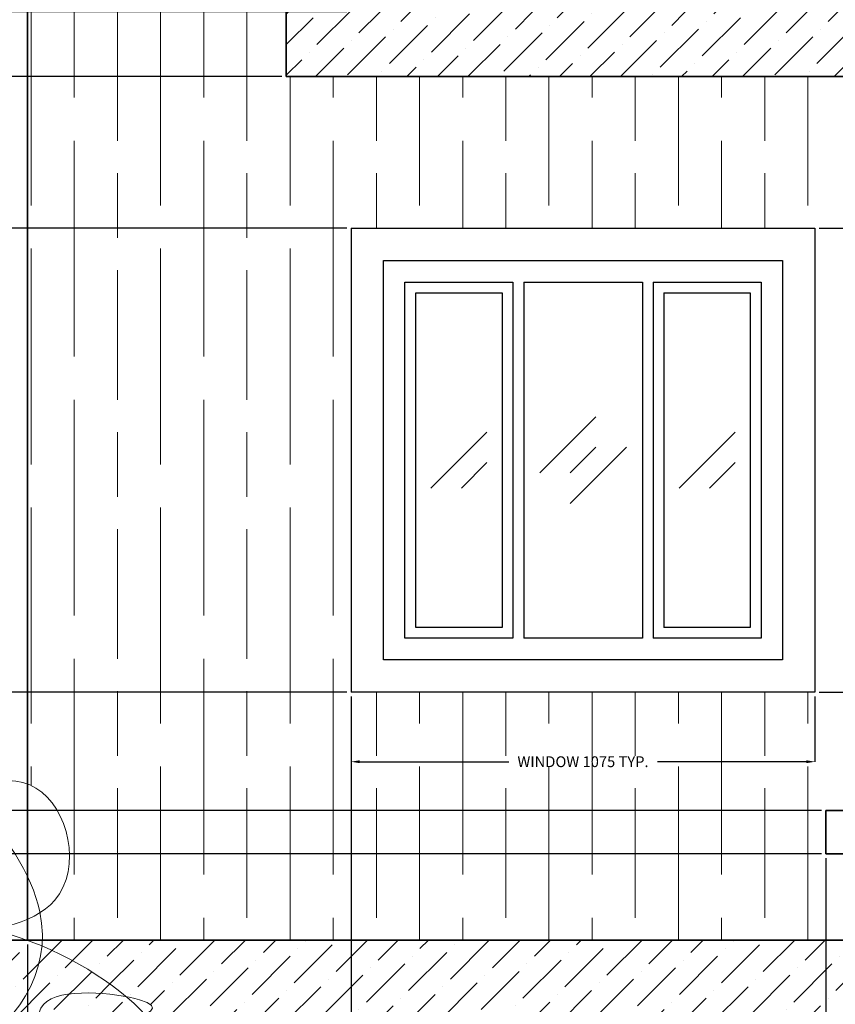
# Model space of a CAD drawing. Units: millimetres. Extents: x -692 to 9639, y -141 to 10345.
# Tile 4 of 19: x 3174 to 5064, y 2699 to 4981. Entities that reach past the tile are written whole.
import ezdxf

# ---------------------------------------------------------------- set-up
doc = ezdxf.new("R2010")
doc.units = ezdxf.units.MM
doc.header["$MEASUREMENT"] = 0
for name, color, linetype, lineweight in [('A-ANNO-DIMS', 2, 'Continuous', 18), ('A-ELEV', 7, 'Continuous', 35), ('A-ELEV-PATT', 8, 'Continuous', 13), ('A-GLAZ', 4, 'Continuous', 25), ('L-PLNT', 3, 'Continuous', 18)]:
    doc.layers.add(name, color=color, linetype=linetype, lineweight=lineweight)
doc.styles.get("Standard").update_dxf_attribs({"font": 'arial.ttf'})
doc.dimstyles.get("Standard").update_dxf_attribs({"dimtxt": 25, "dimasz": 20, "dimexe": 0.18, "dimexo": 10, "dimgap": 10, "dimtad": 0, "dimtih": 1, "dimtoh": 1, "dimdec": 0, "dimzin": 0, "dimdsep": 46, "dimtxsty": 'Standard', "dimcen": 10, "dimadec": 0, "dimazin": 0, "dimtfac": 1, "dimtdec": 0, "dimtofl": 0, "dimtmove": 0, "dimatfit": 3, "dimfxl": 1, "dimtolj": 1, "dimtzin": 0, "dimarcsym": 0})

# ---------------------------------------------------------------- blocks, each defined once
blk = doc.blocks.new('WIN-1075')
for p, q in [((0, 1075), (1075, 1075)), ((0, 1075), (0, 0)), ((1075, 1075), (1075, 0)), ((75, 1000), (1000, 1000)), ((75, 75), (75, 1000)), ((1000, 1000), (1000, 75)), ((125, 950), (375, 950)), ((125, 125), (125, 950)), ((375, 950), (375, 125)), ((400, 950), (400, 125)), ((400, 950), (675, 950)), ((675, 950), (675, 125)), ((700, 950), (700, 125)), ((700, 950), (950, 950)), ((950, 950), (950, 125)), ((150, 150), (150, 925)), ((150, 925), (350, 925)), ((350, 925), (350, 150)), ((725, 925), (725, 150)), ((725, 925), (925, 925)), ((925, 925), (925, 150)), ((567.1, 637.9), (437.1, 507.9)), ((315, 602.5), (185, 472.5)), ((890, 602.5), (760, 472.5)), ((637.9, 567.1), (507.9, 437.1)), ((567.1, 567.1), (507.9, 507.9)), ((315, 531.8), (255.7, 472.5)), ((890, 531.8), (830.7, 472.5)), ((350, 150), (150, 150)), ((925, 150), (725, 150)), ((375, 125), (125, 125)), ((675, 125), (400, 125)), ((950, 125), (700, 125)), ((1000, 75), (75, 75)), ((1075, 0), (0, 0))]:
    blk.add_line(p, q)
blk = doc.blocks.new('*D4')
at = {"layer": 'A-ANNO-DIMS', "color": 0, "lineweight": -2, "transparency": 16777216}
for p, q in [((3941.5, 3412.8), (3941.5, 3261.3)), ((5016.5, 3412.8), (5016.5, 3261.3)), ((3961.5, 3261.5), (4306.8, 3261.5)), ((4996.5, 3261.5), (4651.3, 3261.5))]:
    blk.add_line(p, q, dxfattribs=at)
at = {"layer": 'A-ANNO-DIMS', "color": 0, "lineweight": -3, "transparency": 16777216}
for points in [[(3961.5, 3264.9), (3961.5, 3258.2), (3941.5, 3261.5)], [(4996.5, 3264.9), (4996.5, 3258.2), (5016.5, 3261.5)]]:
    blk.add_solid(points, dxfattribs=at)
at = {"layer": 'Defpoints', "color": 0, "lineweight": -3, "transparency": 16777216}
for p in [(3941.5, 3422.8), (5016.5, 3422.8), (5016.5, 3261.5)]:
    blk.add_point(p, dxfattribs=at)
at = {"layer": 'A-ANNO-DIMS', "color": 0, "transparency": 16777216, "insert": (4479, 3261.5), "char_height": 25, "attachment_point": 5}
blk.add_mtext('\\A1;WINDOW 1075 TYP.', dxfattribs=at)
blk = doc.blocks.new('*D5')
at = {"layer": 'A-ANNO-DIMS', "color": 0, "lineweight": -2, "transparency": 16777216}
for p, q in [((5026.5, 4497.8), (5178, 4497.8)), ((5177.8, 4477.8), (5177.8, 3983)), ((5177.8, 3442.8), (5177.8, 3937.5)), ((5026.5, 3422.8), (5178, 3422.8))]:
    blk.add_line(p, q, dxfattribs=at)
at = {"layer": 'A-ANNO-DIMS', "color": 0, "lineweight": -3, "transparency": 16777216}
for points in [[(5174.5, 4477.8), (5181.1, 4477.8), (5177.8, 4497.8)], [(5174.5, 3442.8), (5181.1, 3442.8), (5177.8, 3422.8)]]:
    blk.add_solid(points, dxfattribs=at)
at = {"layer": 'Defpoints', "color": 0, "lineweight": -3, "transparency": 16777216}
for p in [(5016.5, 4497.8), (5177.8, 4497.8), (5016.5, 3422.8)]:
    blk.add_point(p, dxfattribs=at)
at = {"layer": 'A-ANNO-DIMS', "color": 0, "transparency": 16777216, "insert": (5177.8, 3960.3), "char_height": 25, "attachment_point": 5}
blk.add_mtext('\\A1;1075 TYP.', dxfattribs=at)
blk = doc.blocks.new('*D7')
at = {"layer": 'A-ANNO-DIMS', "color": 0, "lineweight": -2, "transparency": 16777216}
for p, q in [((8481.5, 9848.8), (-649.1, 9848.8)), ((-648.9, 9828.8), (-648.9, 5124.9)), ((-648.9, 375.6), (-648.9, 5079.4)), ((2463.7, 355.6), (-649.1, 355.6))]:
    blk.add_line(p, q, dxfattribs=at)
at = {"layer": 'A-ANNO-DIMS', "color": 0, "lineweight": -3, "transparency": 16777216}
for points in [[(-652.2, 9828.8), (-645.6, 9828.8), (-648.9, 9848.8)], [(-652.2, 375.6), (-645.6, 375.6), (-648.9, 355.6)]]:
    blk.add_solid(points, dxfattribs=at)
at = {"layer": 'Defpoints', "color": 0, "lineweight": -3, "transparency": 16777216}
for p in [(-648.9, 9848.8), (8491.5, 9848.8), (2473.7, 355.6)]:
    blk.add_point(p, dxfattribs=at)
at = {"layer": 'A-ANNO-DIMS', "color": 0, "transparency": 16777216, "insert": (-648.9, 5102.2), "char_height": 25, "attachment_point": 5}
blk.add_mtext('\\A1;9493', dxfattribs=at)
blk = doc.blocks.new('*D37')
at = {"layer": 'A-ANNO-DIMS', "color": 0, "lineweight": -2, "transparency": 16777216}
for p, q in [((3941.5, 3412.8), (3941.5, -124.6)), ((3191.5, 2838.3), (3191.5, -124.6)), ((3211.5, -124.4), (3529.1, -124.4)), ((3921.5, -124.4), (3604, -124.4))]:
    blk.add_line(p, q, dxfattribs=at)
at = {"layer": 'A-ANNO-DIMS', "color": 0, "lineweight": -3, "transparency": 16777216}
for points in [[(3211.5, -121.1), (3211.5, -127.8), (3191.5, -124.4)], [(3921.5, -121.1), (3921.5, -127.8), (3941.5, -124.4)]]:
    blk.add_solid(points, dxfattribs=at)
at = {"layer": 'Defpoints', "color": 0, "lineweight": -3, "transparency": 16777216}
for p in [(3941.5, 3422.8), (3191.5, 2848.3), (3941.5, -124.4)]:
    blk.add_point(p, dxfattribs=at)
at = {"layer": 'A-ANNO-DIMS', "color": 0, "transparency": 16777216, "insert": (3566.5, -124.4), "char_height": 25, "attachment_point": 5}
blk.add_mtext('\\A1;750', dxfattribs=at)
blk = doc.blocks.new('*D38')
at = {"layer": 'A-ANNO-DIMS', "color": 0, "lineweight": -2, "transparency": 16777216}
for p, q in [((3941.5, 3412.8), (3941.5, -124.6)), ((5041.5, 3038.3), (5041.5, -124.6)), ((3961.5, -124.4), (4445.4, -124.4)), ((5021.5, -124.4), (4537.7, -124.4))]:
    blk.add_line(p, q, dxfattribs=at)
at = {"layer": 'A-ANNO-DIMS', "color": 0, "lineweight": -3, "transparency": 16777216}
for points in [[(3961.5, -121.1), (3961.5, -127.8), (3941.5, -124.4)], [(5021.5, -121.1), (5021.5, -127.8), (5041.5, -124.4)]]:
    blk.add_solid(points, dxfattribs=at)
at = {"layer": 'Defpoints', "color": 0, "lineweight": -3, "transparency": 16777216}
for p in [(3941.5, 3422.8), (5041.5, 3048.3), (5041.5, -124.4)]:
    blk.add_point(p, dxfattribs=at)
at = {"layer": 'A-ANNO-DIMS', "color": 0, "transparency": 16777216, "insert": (4491.5, -124.4), "char_height": 25, "attachment_point": 5}
blk.add_mtext('\\A1;1100', dxfattribs=at)
blk = doc.blocks.new('*D39')
at = {"layer": 'A-ANNO-DIMS', "color": 0, "lineweight": -2, "transparency": 16777216}
for p, q in [((5191.5, 3588.3), (5191.5, -124.6)), ((5041.5, 3038.3), (5041.5, -124.6)), ((5061.5, -124.4), (5080.1, -124.4)), ((5171.5, -124.4), (5152.9, -124.4))]:
    blk.add_line(p, q, dxfattribs=at)
at = {"layer": 'A-ANNO-DIMS', "color": 0, "lineweight": -3, "transparency": 16777216}
for points in [[(5061.5, -121.1), (5061.5, -127.8), (5041.5, -124.4)], [(5171.5, -121.1), (5171.5, -127.8), (5191.5, -124.4)]]:
    blk.add_solid(points, dxfattribs=at)
at = {"layer": 'Defpoints', "color": 0, "lineweight": -3, "transparency": 16777216}
for p in [(5191.5, 3598.3), (5041.5, 3048.3), (5191.5, -124.4)]:
    blk.add_point(p, dxfattribs=at)
at = {"layer": 'A-ANNO-DIMS', "color": 0, "transparency": 16777216, "insert": (5116.5, -124.4), "char_height": 25, "attachment_point": 5}
blk.add_mtext('\\A1;150', dxfattribs=at)
blk = doc.blocks.new('*D59')
at = {"layer": 'A-ANNO-DIMS', "color": 0, "lineweight": -2, "transparency": 16777216}
for p, q in [((5031.5, 3048.3), (-649.1, 3048.3)), ((-648.9, 3028.3), (-648.9, 2971)), ((-648.9, 2868.3), (-648.9, 2925.5)), ((3181.5, 2848.3), (-649.1, 2848.3))]:
    blk.add_line(p, q, dxfattribs=at)
at = {"layer": 'A-ANNO-DIMS', "color": 0, "lineweight": -3, "transparency": 16777216}
for points in [[(-652.2, 3028.3), (-645.6, 3028.3), (-648.9, 3048.3)], [(-652.2, 2868.3), (-645.6, 2868.3), (-648.9, 2848.3)]]:
    blk.add_solid(points, dxfattribs=at)
at = {"layer": 'Defpoints', "color": 0, "lineweight": -3, "transparency": 16777216}
for p in [(-648.9, 3048.3), (5041.5, 3048.3), (3191.5, 2848.3)]:
    blk.add_point(p, dxfattribs=at)
at = {"layer": 'A-ANNO-DIMS', "color": 0, "transparency": 16777216, "insert": (-648.9, 2948.3), "char_height": 25, "attachment_point": 5}
blk.add_mtext('\\A1;200', dxfattribs=at)
blk = doc.blocks.new('*D60')
at = {"layer": 'A-ANNO-DIMS', "color": 0, "lineweight": -2, "transparency": 16777216}
for p, q in [((5031.5, 3148.3), (-649.1, 3148.3)), ((-648.9, 3148.3), (-648.9, 3168.3)), ((-648.9, 3168.3), (-628.9, 3168.3)), ((-648.9, 3068.3), (-648.9, 3128.3)), ((5031.5, 3048.3), (-649.1, 3048.3))]:
    blk.add_line(p, q, dxfattribs=at)
at = {"layer": 'A-ANNO-DIMS', "color": 0, "lineweight": -3, "transparency": 16777216}
for points in [[(-652.2, 3128.3), (-645.6, 3128.3), (-648.9, 3148.3)], [(-652.2, 3068.3), (-645.6, 3068.3), (-648.9, 3048.3)]]:
    blk.add_solid(points, dxfattribs=at)
at = {"layer": 'Defpoints', "color": 0, "lineweight": -3, "transparency": 16777216}
for p in [(-648.9, 3148.3), (5041.5, 3148.3), (5041.5, 3048.3)]:
    blk.add_point(p, dxfattribs=at)
at = {"layer": 'A-ANNO-DIMS', "color": 0, "transparency": 16777216, "insert": (-592.5, 3168.3), "char_height": 25, "attachment_point": 5}
blk.add_mtext('\\A1;100', dxfattribs=at)
blk = doc.blocks.new('*D61')
at = {"layer": 'A-ANNO-DIMS', "color": 0, "lineweight": -2, "transparency": 16777216}
for p, q in [((3931.5, 3422.8), (-649.1, 3422.8)), ((-648.9, 3402.8), (-648.9, 3308.3)), ((-648.9, 3168.3), (-648.9, 3262.8)), ((5031.5, 3148.3), (-649.1, 3148.3))]:
    blk.add_line(p, q, dxfattribs=at)
at = {"layer": 'A-ANNO-DIMS', "color": 0, "lineweight": -3, "transparency": 16777216}
for points in [[(-652.2, 3402.8), (-645.6, 3402.8), (-648.9, 3422.8)], [(-652.2, 3168.3), (-645.6, 3168.3), (-648.9, 3148.3)]]:
    blk.add_solid(points, dxfattribs=at)
at = {"layer": 'Defpoints', "color": 0, "lineweight": -3, "transparency": 16777216}
for p in [(-648.9, 3422.8), (3941.5, 3422.8), (5041.5, 3148.3)]:
    blk.add_point(p, dxfattribs=at)
at = {"layer": 'A-ANNO-DIMS', "color": 0, "transparency": 16777216, "insert": (-648.9, 3285.5), "char_height": 25, "attachment_point": 5}
blk.add_mtext('\\A1;274.5', dxfattribs=at)
blk = doc.blocks.new('*D62')
at = {"layer": 'A-ANNO-DIMS', "color": 0, "lineweight": -2, "transparency": 16777216}
for p, q in [((3781.5, 4848.8), (-649.1, 4848.8)), ((-648.9, 4828.8), (-648.9, 4696)), ((-648.9, 4517.8), (-648.9, 4650.5)), ((3931.5, 4497.8), (-649.1, 4497.8))]:
    blk.add_line(p, q, dxfattribs=at)
at = {"layer": 'A-ANNO-DIMS', "color": 0, "lineweight": -3, "transparency": 16777216}
for points in [[(-652.2, 4828.8), (-645.6, 4828.8), (-648.9, 4848.8)], [(-652.2, 4517.8), (-645.6, 4517.8), (-648.9, 4497.8)]]:
    blk.add_solid(points, dxfattribs=at)
at = {"layer": 'Defpoints', "color": 0, "lineweight": -3, "transparency": 16777216}
for p in [(-648.9, 4848.8), (3791.5, 4848.8), (3941.5, 4497.8)]:
    blk.add_point(p, dxfattribs=at)
at = {"layer": 'A-ANNO-DIMS', "color": 0, "transparency": 16777216, "insert": (-648.9, 4673.3), "char_height": 25, "attachment_point": 5}
blk.add_mtext('\\A1;351', dxfattribs=at)
blk = doc.blocks.new('*D63')
at = {"layer": 'A-ANNO-DIMS', "color": 0, "lineweight": -2, "transparency": 16777216}
for p, q in [((3931.5, 4998.8), (-649.1, 4998.8)), ((-648.9, 4978.8), (-648.9, 4946.5)), ((-648.9, 4868.8), (-648.9, 4901)), ((3781.5, 4848.8), (-649.1, 4848.8))]:
    blk.add_line(p, q, dxfattribs=at)
at = {"layer": 'A-ANNO-DIMS', "color": 0, "lineweight": -3, "transparency": 16777216}
for points in [[(-652.2, 4978.8), (-645.6, 4978.8), (-648.9, 4998.8)], [(-652.2, 4868.8), (-645.6, 4868.8), (-648.9, 4848.8)]]:
    blk.add_solid(points, dxfattribs=at)
at = {"layer": 'Defpoints', "color": 0, "lineweight": -3, "transparency": 16777216}
for p in [(-648.9, 4998.8), (3941.5, 4998.8), (3791.5, 4848.8)]:
    blk.add_point(p, dxfattribs=at)
at = {"layer": 'A-ANNO-DIMS', "color": 0, "transparency": 16777216, "insert": (-648.9, 4923.8), "char_height": 25, "attachment_point": 5}
blk.add_mtext('\\A1;150', dxfattribs=at)

msp = doc.modelspace()

# ---------------------------------------------------------------- hatches: boundary and pattern name
at = {"layer": 'A-ELEV-PATT'}
h = msp.add_hatch(dxfattribs=at)
h.set_pattern_fill('GOST_WOOD', color=256, scale=50)
h.set_pattern_definition([(90, (0, 0), (300, -2e-14), [500, -100]), (90, (100, -100), (300, -2e-14), [300, -75, 150, -75]), (90, (200, -250), (300, -2e-14), [500, -100])])
edge = h.paths.add_edge_path()
edge.add_line((5191.547, 8748.772), (3791.547, 8748.772))
edge.add_line((3791.547, 8748.772), (3791.547, 8848.772))
edge.add_line((3791.547, 8848.772), (5191.547, 8848.772))
edge.add_line((5191.547, 8848.772), (5191.547, 9348.772))
edge.add_line((5191.547, 9348.772), (4755.992, 9348.772))
edge.add_line((4755.992, 9348.772), (4755.854, 9348.465))
edge.add_line((4755.854, 9348.465), (4755.734, 9348.772))
edge.add_line((4755.734, 9348.772), (4053.129, 9348.772))
edge.add_line((4053.129, 9348.772), (4052.99, 9348.465))
edge.add_line((4052.99, 9348.465), (4052.871, 9348.772))
edge.add_line((4052.871, 9348.772), (3701.731, 9348.772))
edge.add_line((3701.731, 9348.772), (3701.593, 9348.465))
edge.add_line((3701.593, 9348.465), (3701.474, 9348.772))
edge.add_line((3701.474, 9348.772), (3368.199, 9348.772))
edge.add_line((3368.199, 9348.772), (3368.061, 9348.465))
edge.add_line((3368.061, 9348.465), (3367.942, 9348.772))
edge.add_line((3367.942, 9348.772), (3191.547, 9348.772))
edge.add_line((3191.547, 9348.772), (3191.547, 3210.058))
edge.add_spline(control_points=[(3191.547, 3210.058), (3198.467, 3207.5), (3283.859, 3166.656), (3324.053, 2995.08), (3234.02, 2920.058), (3220.783, 2911.684)], knot_values=[13649.89756952, 13649.89756952, 13649.89756952, 13649.89756952, 13672.14990348, 13935.42377748, 13974.4426778, 13974.4426778, 13974.4426778, 13974.4426778], degree=3, periodic=0)
edge.add_spline(control_points=[(3220.783, 2911.684), (3225.148, 2890.107), (3226.864, 2868.931), (3226.144, 2848.27)], knot_values=[8828.69997321, 8828.69997321, 8828.69997321, 8828.69997321, 8890.6429847, 8890.6429847, 8890.6429847, 8890.6429847], degree=3, periodic=0)
edge.add_line((3226.144, 2848.27), (5191.547, 2848.27))
edge.add_line((5191.547, 2848.27), (5191.547, 3048.27))
edge.add_line((5191.547, 3048.27), (5041.547, 3048.27))
edge.add_line((5041.547, 3048.27), (5041.547, 3148.27))
edge.add_line((5041.547, 3148.27), (5091.547, 3148.27))
edge.add_line((5091.547, 3148.27), (5091.547, 3598.27))
edge.add_line((5091.547, 3598.27), (5191.547, 3598.27))
edge.add_line((5191.547, 3598.27), (5191.547, 4848.772))
edge.add_line((5191.547, 4848.772), (3791.547, 4848.772))
edge.add_line((3791.547, 4848.772), (3791.547, 6848.772))
edge.add_line((3791.547, 6848.772), (5091.547, 6848.772))
edge.add_line((5091.547, 6848.772), (5091.547, 7298.772))
edge.add_line((5091.547, 7298.772), (5191.547, 7298.772))
edge.add_line((5191.547, 7298.772), (5191.547, 8748.772))
h.paths.add_polyline_path([(5016.547, 8198.772), (5016.547, 7123.772), (3941.547, 7123.772), (3941.547, 8198.772)], flags=16)
h.paths.add_polyline_path([(4941.547, 8123.772), (4941.547, 7198.772), (4016.547, 7198.772), (4016.547, 8123.772)], flags=0)
h.paths.add_polyline_path([(4616.547, 8073.772), (4616.547, 7248.772), (4341.547, 7248.772), (4341.547, 8073.772)], flags=0)
h.paths.add_polyline_path([(4641.547, 8073.772), (4891.547, 8073.772), (4891.547, 7248.772), (4641.547, 7248.772)], flags=0)
h.paths.add_polyline_path([(4666.547, 8048.772), (4866.547, 8048.772), (4866.547, 7273.772), (4666.547, 7273.772)], flags=0)
h.paths.add_polyline_path([(4316.547, 8073.772), (4316.547, 7248.772), (4066.547, 7248.772), (4066.547, 8073.772)], flags=0)
h.paths.add_polyline_path([(4291.547, 8048.772), (4291.547, 7273.772), (4091.547, 7273.772), (4091.547, 8048.772)], flags=0)
h.paths.add_polyline_path([(5016.547, 4497.772), (5016.547, 3422.772), (3941.547, 3422.772), (3941.547, 4497.772)], flags=16)
h.paths.add_polyline_path([(4941.547, 4422.772), (4941.547, 3497.772), (4016.547, 3497.772), (4016.547, 4422.772)], flags=0)
h.paths.add_polyline_path([(4616.547, 4372.772), (4616.547, 3547.772), (4341.547, 3547.772), (4341.547, 4372.772)], flags=0)
h.paths.add_polyline_path([(4641.547, 4372.772), (4891.547, 4372.772), (4891.547, 3547.772), (4641.547, 3547.772)], flags=0)
h.paths.add_polyline_path([(4316.547, 4372.772), (4316.547, 3547.772), (4066.547, 3547.772), (4066.547, 4372.772)], flags=0)
h.paths.add_polyline_path([(4666.547, 4347.772), (4866.547, 4347.772), (4866.547, 3572.772), (4666.547, 3572.772)], flags=0)
h.paths.add_polyline_path([(4291.547, 4347.772), (4291.547, 3572.772), (4091.547, 3572.772), (4091.547, 4347.772)], flags=0)
h = msp.add_hatch(dxfattribs=at)
h.set_pattern_fill('ANSI36', color=256, scale=400)
h.paths.add_polyline_path([(8691.547, 6848.772), (3791.547, 6848.772), (3791.547, 4848.772), (8691.547, 4848.772), (8691.547, 4998.772), (3941.547, 4998.772), (3941.547, 6698.772), (8691.547, 6698.772)])
h = msp.add_hatch(dxfattribs=at)
h.set_pattern_fill('ANSI36', color=256, scale=400)
edge = h.paths.add_edge_path()
edge.add_spline(control_points=[(3173.746, 2309.965), (3085.901, 2332.226), (2969.139, 2424.713), (2876.436, 2493.45)], knot_values=[20955.88576955, 20955.88576955, 20955.88576955, 20955.88576955, 21219.85539585, 21219.85539585, 21219.85539585, 21219.85539585], degree=3, periodic=0)
edge.add_spline(control_points=[(2876.436, 2493.45), (2855.134, 2468.311), (2819.135, 2451.154), (2773.746, 2440.514)], knot_values=[5238.08213467, 5238.08213467, 5238.08213467, 5238.08213467, 5382.8513026, 5382.8513026, 5382.8513026, 5382.8513026], degree=3, periodic=0)
edge.add_line((2773.746, 2440.514), (2773.746, 2354.397))
edge.add_spline(control_points=[(2773.746, 2354.397), (2777.278, 2343.918), (2780.812, 2333.449), (2784.279, 2323.093)], knot_values=[20514.20511429, 20514.20511429, 20514.20511429, 20514.20511429, 20537.39604293, 20537.39604293, 20537.39604293, 20537.39604293], degree=3, periodic=0)
edge.add_spline(control_points=[(2784.279, 2323.093), (2849.257, 2305.468), (3007.384, 2255.171), (2928.441, 2185.016), (2819.76, 2148.371)], knot_values=[1896.27813718, 1896.27813718, 1896.27813718, 1896.27813718, 2077.70067144, 2424.51760392, 2424.51760392, 2424.51760392, 2424.51760392], degree=3, periodic=0)
edge.add_spline(control_points=[(2819.76, 2148.371), (2817.899, 2146.748), (2815.52, 2145.926), (2812.57, 2145.987)], knot_values=[20304.87329269, 20304.87329269, 20304.87329269, 20304.87329269, 20326.21847821, 20326.21847821, 20326.21847821, 20326.21847821], degree=3, periodic=0)
edge.add_spline(control_points=[(2812.57, 2145.987), (2800.291, 2141.985), (2787.329, 2138.102), (2773.746, 2134.363)], knot_values=[1850.39591646, 1850.39591646, 1850.39591646, 1850.39591646, 1888.716341, 1888.716341, 1888.716341, 1888.716341], degree=3, periodic=0)
edge.add_line((2773.746, 2134.363), (2773.746, 855.575))
edge.add_line((2773.746, 855.575), (3173.746, 855.575))
edge.add_line((3173.746, 855.575), (3173.746, 2309.965))
edge = h.paths.add_edge_path()
edge.add_spline(control_points=[(3420.651, 2717.101), (3368.378, 2761.363), (3299.425, 2803.396), (3225.3, 2834.508)], knot_values=[12552.99587302, 12552.99587302, 12552.99587302, 12552.99587302, 12712.02358035, 12712.02358035, 12712.02358035, 12712.02358035], degree=3, periodic=0)
edge.add_spline(control_points=[(3225.3, 2834.508), (3218.267, 2754.576), (3174.644, 2682.922), (3107.112, 2626.403)], knot_values=[8572.46293399, 8572.46293399, 8572.46293399, 8572.46293399, 8814.86919927, 8814.86919927, 8814.86919927, 8814.86919927], degree=3, periodic=0)
edge.add_spline(control_points=[(3107.112, 2626.403), (3129.755, 2627.593), (3152.034, 2628.996), (3173.746, 2630.586)], knot_values=[10558.19039557, 10558.19039557, 10558.19039557, 10558.19039557, 10599.03834951, 10599.03834951, 10599.03834951, 10599.03834951], degree=3, periodic=0)
edge.add_line((3173.746, 2630.586), (3173.746, 2648.27))
edge.add_line((3173.746, 2648.27), (3219.774, 2648.27))
edge.add_spline(control_points=[(3219.774, 2648.27), (3215.509, 2669.279), (3223.352, 2735.229), (3357.845, 2728.872), (3420.651, 2717.101)], knot_values=[11042.13010686, 11042.13010686, 11042.13010686, 11042.13010686, 11110.4948836, 11298.41454305, 11298.41454305, 11298.41454305, 11298.41454305], degree=3, periodic=0)
edge = h.paths.add_edge_path()
edge.add_spline(control_points=[(3107.112, 2626.403), (3174.644, 2682.922), (3218.267, 2754.576), (3225.3, 2834.508)], knot_values=[8572.46293399, 8572.46293399, 8572.46293399, 8572.46293399, 8814.86919927, 8814.86919927, 8814.86919927, 8814.86919927], degree=3, periodic=0)
edge.add_spline(control_points=[(3225.3, 2834.508), (3213.709, 2839.374), (3201.991, 2843.972), (3190.19, 2848.27)], knot_values=[12712.02358035, 12712.02358035, 12712.02358035, 12712.02358035, 12736.8923557, 12736.8923557, 12736.8923557, 12736.8923557], degree=3, periodic=0)
edge.add_line((3190.19, 2848.27), (2928.387, 2848.27))
edge.add_spline(control_points=[(2928.387, 2848.27), (2886.081, 2816.098), (2840.884, 2784.767), (2798.089, 2758.256)], knot_values=[14939.29716066, 14939.29716066, 14939.29716066, 14939.29716066, 15046.25935392, 15046.25935392, 15046.25935392, 15046.25935392], degree=3, periodic=0)
edge.add_spline(control_points=[(2798.089, 2758.256), (2836.427, 2711.897), (2866.292, 2664.879), (2883.022, 2622.327)], knot_values=[5561.23366662, 5561.23366662, 5561.23366662, 5561.23366662, 5704.57044689, 5704.57044689, 5704.57044689, 5704.57044689], degree=3, periodic=0)
edge.add_spline(control_points=[(2883.022, 2622.327), (2956.927, 2620.92), (3033.919, 2622.554), (3107.112, 2626.403)], knot_values=[10426.14846168, 10426.14846168, 10426.14846168, 10426.14846168, 10558.19039557, 10558.19039557, 10558.19039557, 10558.19039557], degree=3, periodic=0)
edge = h.paths.add_edge_path()
edge.add_spline(control_points=[(3173.746, 2630.586), (3152.034, 2628.996), (3129.755, 2627.593), (3107.112, 2626.403)], knot_values=[10558.19039557, 10558.19039557, 10558.19039557, 10558.19039557, 10599.03834951, 10599.03834951, 10599.03834951, 10599.03834951], degree=3, periodic=0)
edge.add_spline(control_points=[(3107.112, 2626.403), (3049.969, 2578.578), (2975.708, 2541.59), (2892.012, 2519.592)], knot_values=[8367.34849038, 8367.34849038, 8367.34849038, 8367.34849038, 8572.46293399, 8572.46293399, 8572.46293399, 8572.46293399], degree=3, periodic=0)
edge.add_spline(control_points=[(2892.012, 2519.592), (2888.384, 2510.058), (2883.137, 2501.359), (2876.436, 2493.45)], knot_values=[5382.8513026, 5382.8513026, 5382.8513026, 5382.8513026, 5428.39625745, 5428.39625745, 5428.39625745, 5428.39625745], degree=3, periodic=0)
edge.add_spline(control_points=[(2876.436, 2493.45), (2969.139, 2424.713), (3085.901, 2332.226), (3173.746, 2309.965)], knot_values=[20955.88576955, 20955.88576955, 20955.88576955, 20955.88576955, 21219.85539585, 21219.85539585, 21219.85539585, 21219.85539585], degree=3, periodic=0)
edge.add_line((3173.746, 2309.965), (3173.746, 2630.586))
edge = h.paths.add_edge_path(flags=17)
edge.add_spline(control_points=[(2819.76, 2148.371), (2928.441, 2185.016), (3007.384, 2255.171), (2849.257, 2305.468), (2784.279, 2323.093)], knot_values=[1896.27813718, 1896.27813718, 1896.27813718, 1896.27813718, 2243.09506965, 2424.51760392, 2424.51760392, 2424.51760392, 2424.51760392], degree=3, periodic=0)
edge.add_spline(control_points=[(2784.279, 2323.093), (2812.387, 2239.151), (2836.152, 2162.664), (2819.76, 2148.371)], knot_values=[20326.21847821, 20326.21847821, 20326.21847821, 20326.21847821, 20514.20511429, 20514.20511429, 20514.20511429, 20514.20511429], degree=3, periodic=0)
edge = h.paths.add_edge_path(flags=17)
edge.add_spline(control_points=[(2819.76, 2148.371), (2836.152, 2162.664), (2812.387, 2239.151), (2784.279, 2323.093)], knot_values=[20326.21847821, 20326.21847821, 20326.21847821, 20326.21847821, 20514.20511429, 20514.20511429, 20514.20511429, 20514.20511429], degree=3, periodic=0)
edge.add_spline(control_points=[(2784.279, 2323.093), (2780.798, 2324.038), (2777.286, 2324.983), (2773.746, 2325.93)], knot_values=[2424.51760392, 2424.51760392, 2424.51760392, 2424.51760392, 2434.23800618, 2434.23800618, 2434.23800618, 2434.23800618], degree=3, periodic=0)
edge.add_line((2773.746, 2325.93), (2773.746, 2166.486))
edge.add_spline(control_points=[(2773.746, 2166.486), (2790.303, 2153.967), (2803.9, 2146.166), (2812.57, 2145.987)], knot_values=[20242.12265912, 20242.12265912, 20242.12265912, 20242.12265912, 20304.87329269, 20304.87329269, 20304.87329269, 20304.87329269], degree=3, periodic=0)
edge.add_spline(control_points=[(2812.57, 2145.987), (2814.994, 2146.777), (2817.39, 2147.572), (2819.76, 2148.371)], knot_values=[1888.716341, 1888.716341, 1888.716341, 1888.716341, 1896.27813718, 1896.27813718, 1896.27813718, 1896.27813718], degree=3, periodic=0)
edge = h.paths.add_edge_path()
edge.add_spline(control_points=[(2892.012, 2519.592), (2893.653, 2523.907), (2902.094, 2552.818), (2896.12, 2589.012), (2883.022, 2622.327)], knot_values=[5428.39625745, 5428.39625745, 5428.39625745, 5428.39625745, 5449.01011401, 5561.23366662, 5561.23366662, 5561.23366662, 5561.23366662], degree=3, periodic=0)
edge.add_spline(control_points=[(2883.022, 2622.327), (2845.501, 2623.042), (2808.775, 2624.54), (2773.746, 2626.93)], knot_values=[10359.11175247, 10359.11175247, 10359.11175247, 10359.11175247, 10426.14846168, 10426.14846168, 10426.14846168, 10426.14846168], degree=3, periodic=0)
edge.add_line((2773.746, 2626.93), (2773.746, 2561.8))
edge.add_spline(control_points=[(2773.746, 2561.8), (2795.257, 2551.206), (2822.448, 2532.82), (2853.096, 2510.59)], knot_values=[20841.44589883, 20841.44589883, 20841.44589883, 20841.44589883, 20933.19502211, 20933.19502211, 20933.19502211, 20933.19502211], degree=3, periodic=0)
edge.add_spline(control_points=[(2853.096, 2510.59), (2866.269, 2513.232), (2879.25, 2516.238), (2892.012, 2519.592)], knot_values=[8336.07392909, 8336.07392909, 8336.07392909, 8336.07392909, 8367.34849038, 8367.34849038, 8367.34849038, 8367.34849038], degree=3, periodic=0)
edge = h.paths.add_edge_path(flags=17)
edge.add_spline(control_points=[(2892.012, 2519.592), (2975.708, 2541.59), (3049.969, 2578.578), (3107.112, 2626.403)], knot_values=[8367.34849038, 8367.34849038, 8367.34849038, 8367.34849038, 8572.46293399, 8572.46293399, 8572.46293399, 8572.46293399], degree=3, periodic=0)
edge.add_spline(control_points=[(3107.112, 2626.403), (3033.919, 2622.554), (2956.927, 2620.92), (2883.022, 2622.327)], knot_values=[10426.14846168, 10426.14846168, 10426.14846168, 10426.14846168, 10558.19039557, 10558.19039557, 10558.19039557, 10558.19039557], degree=3, periodic=0)
edge.add_spline(control_points=[(2883.022, 2622.327), (2896.12, 2589.012), (2902.094, 2552.818), (2893.653, 2523.907), (2892.012, 2519.592)], knot_values=[5428.39625745, 5428.39625745, 5428.39625745, 5428.39625745, 5540.61981006, 5561.23366662, 5561.23366662, 5561.23366662, 5561.23366662], degree=3, periodic=0)
edge = h.paths.add_edge_path()
edge.add_spline(control_points=[(2773.746, 2440.514), (2819.135, 2451.154), (2855.134, 2468.311), (2876.436, 2493.45)], knot_values=[5238.08213467, 5238.08213467, 5238.08213467, 5238.08213467, 5382.8513026, 5382.8513026, 5382.8513026, 5382.8513026], degree=3, periodic=0)
edge.add_spline(control_points=[(2876.436, 2493.45), (2868.467, 2499.359), (2860.676, 2505.092), (2853.096, 2510.59)], knot_values=[20933.19502211, 20933.19502211, 20933.19502211, 20933.19502211, 20955.88576955, 20955.88576955, 20955.88576955, 20955.88576955], degree=3, periodic=0)
edge.add_spline(control_points=[(2853.096, 2510.59), (2827.314, 2505.418), (2800.796, 2501.637), (2773.746, 2499.359)], knot_values=[8274.86392127, 8274.86392127, 8274.86392127, 8274.86392127, 8336.07392909, 8336.07392909, 8336.07392909, 8336.07392909], degree=3, periodic=0)
edge.add_line((2773.746, 2499.359), (2773.746, 2440.514))
edge = h.paths.add_edge_path()
edge.add_spline(control_points=[(2883.022, 2622.327), (2866.292, 2664.879), (2836.427, 2711.897), (2798.089, 2758.256)], knot_values=[5561.23366662, 5561.23366662, 5561.23366662, 5561.23366662, 5704.57044689, 5704.57044689, 5704.57044689, 5704.57044689], degree=3, periodic=0)
edge.add_spline(control_points=[(2798.089, 2758.256), (2789.874, 2753.166), (2781.747, 2748.254), (2773.746, 2743.548)], knot_values=[15046.25935392, 15046.25935392, 15046.25935392, 15046.25935392, 15066.79294618, 15066.79294618, 15066.79294618, 15066.79294618], degree=3, periodic=0)
edge.add_line((2773.746, 2743.548), (2773.746, 2626.93))
edge.add_spline(control_points=[(2773.746, 2626.93), (2808.775, 2624.54), (2845.501, 2623.042), (2883.022, 2622.327)], knot_values=[10359.11175247, 10359.11175247, 10359.11175247, 10359.11175247, 10426.14846168, 10426.14846168, 10426.14846168, 10426.14846168], degree=3, periodic=0)
edge = h.paths.add_edge_path()
edge.add_spline(control_points=[(2798.089, 2758.256), (2840.884, 2784.767), (2886.081, 2816.098), (2928.387, 2848.27)], knot_values=[14939.29716066, 14939.29716066, 14939.29716066, 14939.29716066, 15046.25935392, 15046.25935392, 15046.25935392, 15046.25935392], degree=3, periodic=0)
edge.add_line((2928.387, 2848.27), (2773.746, 2848.27))
edge.add_line((2773.746, 2848.27), (2773.746, 2786.349))
edge.add_spline(control_points=[(2773.746, 2786.349), (2782.183, 2777.04), (2790.311, 2767.662), (2798.089, 2758.256)], knot_values=[5704.57044689, 5704.57044689, 5704.57044689, 5704.57044689, 5733.65273084, 5733.65273084, 5733.65273084, 5733.65273084], degree=3, periodic=0)
edge = h.paths.add_edge_path()
edge.add_spline(control_points=[(3463.702, 2676.006), (3451.141, 2689.747), (3436.681, 2703.529), (3420.651, 2717.101)], knot_values=[12504.23047843, 12504.23047843, 12504.23047843, 12504.23047843, 12552.99587302, 12552.99587302, 12552.99587302, 12552.99587302], degree=3, periodic=0)
edge.add_spline(control_points=[(3420.651, 2717.101), (3357.845, 2728.872), (3223.352, 2735.229), (3215.509, 2669.279), (3219.774, 2648.27)], knot_values=[11042.13010686, 11042.13010686, 11042.13010686, 11042.13010686, 11230.04976631, 11298.41454305, 11298.41454305, 11298.41454305, 11298.41454305], degree=3, periodic=0)
edge.add_line((3219.774, 2648.27), (3341.426, 2648.27))
edge.add_spline(control_points=[(3341.426, 2648.27), (3397.595, 2656.506), (3440.895, 2666.057), (3463.702, 2676.006)], knot_values=[10715.9300286, 10715.9300286, 10715.9300286, 10715.9300286, 10852.53626518, 10852.53626518, 10852.53626518, 10852.53626518], degree=3, periodic=0)
edge = h.paths.add_edge_path()
edge.add_spline(control_points=[(2853.096, 2510.59), (2822.448, 2532.82), (2795.257, 2551.206), (2773.746, 2561.8)], knot_values=[20841.44589883, 20841.44589883, 20841.44589883, 20841.44589883, 20933.19502211, 20933.19502211, 20933.19502211, 20933.19502211], degree=3, periodic=0)
edge.add_line((2773.746, 2561.8), (2773.746, 2499.359))
edge.add_spline(control_points=[(2773.746, 2499.359), (2800.796, 2501.637), (2827.314, 2505.418), (2853.096, 2510.59)], knot_values=[8274.86392127, 8274.86392127, 8274.86392127, 8274.86392127, 8336.07392909, 8336.07392909, 8336.07392909, 8336.07392909], degree=3, periodic=0)
h = msp.add_hatch(dxfattribs=at)
h.set_pattern_fill('ANSI36', color=256, scale=400)
edge = h.paths.add_edge_path()
edge.add_line((5773.746, 2848.27), (3226.144, 2848.27))
edge.add_spline(control_points=[(3226.144, 2848.27), (3225.984, 2843.657), (3225.702, 2839.069), (3225.3, 2834.508)], knot_values=[8814.86919927, 8814.86919927, 8814.86919927, 8814.86919927, 8828.69997321, 8828.69997321, 8828.69997321, 8828.69997321], degree=3, periodic=0)
edge.add_spline(control_points=[(3225.3, 2834.508), (3299.425, 2803.396), (3368.378, 2761.363), (3420.651, 2717.101)], knot_values=[12552.99587302, 12552.99587302, 12552.99587302, 12552.99587302, 12712.02358035, 12712.02358035, 12712.02358035, 12712.02358035], degree=3, periodic=0)
edge.add_spline(control_points=[(3420.651, 2717.101), (3432.322, 2714.914), (3488.975, 2701.706), (3489.525, 2687.271), (3463.702, 2676.006)], knot_values=[10852.53626518, 10852.53626518, 10852.53626518, 10852.53626518, 10887.45464539, 11042.13010686, 11042.13010686, 11042.13010686, 11042.13010686], degree=3, periodic=0)
edge.add_spline(control_points=[(3463.702, 2676.006), (3472.194, 2666.716), (3479.817, 2657.445), (3486.469, 2648.27)], knot_values=[12471.26094935, 12471.26094935, 12471.26094935, 12471.26094935, 12504.23047843, 12504.23047843, 12504.23047843, 12504.23047843], degree=3, periodic=0)
edge.add_line((3486.469, 2648.27), (5373.746, 2648.27))
edge.add_line((5373.746, 2648.27), (5373.746, 855.575))
edge.add_line((5373.746, 855.575), (5773.746, 855.575))
edge.add_line((5773.746, 855.575), (5773.746, 2848.27))

# ---------------------------------------------------------------- linework, layer by layer
at = {"layer": 'A-ELEV'}
for p, q in [((3191.547, 2848.27), (3191.547, 9348.772)), ((3791.547, 4848.772), (3791.547, 6848.772)), ((3791.547, 4848.772), (8691.547, 4848.772)), ((5041.547, 3048.27), (5041.547, 3148.27)), ((5041.547, 3148.27), (5191.547, 3148.27)), ((5191.547, 3048.27), (5041.547, 3048.27)), ((2773.746, 2848.27), (5773.746, 2848.27))]:
    msp.add_line(p, q, dxfattribs=at)
at = {"layer": 'L-PLNT'}
msp.add_open_spline([(2323.333, 2214.265), (2305.649, 2163.243), (2257.888, 2025.445), (1935.117, 1924.822), (1413.715, 2416.586), (2206.705, 1935.154), (3264.488, 2224.597), (2555.092, 2370.602), (2159.771, 2527.783), (2008.053, 1993.707), (1823.12, 2332.645), (1174.123, 2625.596), (1944.245, 2620.173), (2297.612, 2431.636), (3340.282, 2329.714), (2122.894, 3461.216), (2087.569, 2088.062), (1584.671, 3289.033), (2501.939, 2207.058), (3524.445, 2766.924), (2798.31, 3455.317), (2706.153, 2954.832), (2166.187, 2516.526), (3968.598, 2664.724), (2990, 2769.255), (3688.565, 2108.449), (2982.144, 2461.359), (3771.592, 2459.928), (3182.433, 2965.822), (2527.115, 2819.368), (3221.379, 3433.367), (3370.439, 2797.07), (2591.814, 2891.377), (3329.128, 3168.682), (2633.805, 2580.308), (2320.472, 2701.322), (1352.991, 2495.29), (1929.878, 2444.347), (2406.24, 1895.881), (1637.78, 2788.225), (1673.077, 2130.341), (1834.638, 1713.755), (2155.278, 2063.673), (2496.635, 2611.137), (2362.564, 2025.688), (2789.19, 1894.041), (2353.111, 2630.053), (3000.854, 1872.269), (2485.666, 2949.85), (3219.61, 2114.193), (3315.543, 2405.105), (3339.585, 2478.009)], degree=3, knots=[0, 0, 0, 0, 156.01346293, 421.35741543, 891.47725045, 1326.49022079, 2243.09506965, 2561.11240616, 3034.23136561, 3344.76171519, 3437.70824639, 4024.35592839, 4525.63722229, 4755.92435047, 5449.01011401, 6226.81953685, 6823.80489855, 7287.95261826, 8086.77706947, 8892.28439463, 9398.99039818, 9802.71434696, 10041.58770662, 11007.21172666, 11230.04976631, 11694.3239388, 11960.50265147, 12274.78503374, 12794.79981033, 13145.39931196, 13672.14990348, 13935.42377748, 14348.98904743, 14621.34829061, 15077.00752658, 15638.15277437, 16264.82873645, 16548.19934354, 16952.30560132, 17525.13857657, 17920.46774586, 18221.89473837, 18637.38469135, 19024.43489898, 19426.39819861, 19566.65499761, 19968.27543453, 20304.87329269, 20724.59660574, 21299.21696159, 21491.37708517, 21491.37708517, 21491.37708517, 21491.37708517], dxfattribs=at)

# ---------------------------------------------------------------- block references
at = {"layer": 'A-GLAZ'}
msp.add_blockref('WIN-1075', (3941.547, 3422.772), dxfattribs=at)

# ---------------------------------------------------------------- dimensions: what is measured, and where the dimension line sits
at = {"layer": 'A-ANNO-DIMS'}
for base, p1, p2, override, picture, middle in [((-648.912, 9848.772), (2473.746, 355.575), (8491.547, 9848.772), {"dimdec": 0, "dimlfac": 1, "dimrnd": 0, "dimzin": 0, "dimdsep": 46, "dimlunit": 2}, '*D7', (-648.912, 5102.173)), ((-648.912, 4998.772), (3791.547, 4848.772), (3941.547, 4998.772), {"dimdec": 0, "dimlfac": 1, "dimrnd": 0, "dimzin": 0, "dimdsep": 46, "dimlunit": 2}, '*D63', (-648.912, 4923.772)), ((-648.912, 4848.772), (3941.547, 4497.772), (3791.547, 4848.772), {"dimdec": 0, "dimlfac": 1, "dimrnd": 0, "dimzin": 0, "dimdsep": 46, "dimlunit": 2}, '*D62', (-648.912, 4673.272)), ((-648.912, 3422.772), (5041.547, 3148.27), (3941.547, 3422.772), {"dimdec": 1, "dimlfac": 1, "dimrnd": 0, "dimzin": 0, "dimdsep": 46, "dimlunit": 2}, '*D61', (-648.912, 3285.521)), ((-648.912, 3148.27), (5041.547, 3048.27), (5041.547, 3148.27), {"dimdec": 0, "dimlfac": 1, "dimrnd": 0, "dimzin": 0, "dimdsep": 46, "dimlunit": 2}, '*D60', (-592.514, 3168.27)), ((-648.912, 3048.27), (3191.547, 2848.27), (5041.547, 3048.27), {"dimdec": 0, "dimlfac": 1, "dimrnd": 0, "dimzin": 0, "dimdsep": 46, "dimlunit": 2}, '*D59', (-648.912, 2948.27))]:
    dim = msp.add_linear_dim(base=base, p1=p1, p2=p2, angle=90, dimstyle='Standard', override=override, dxfattribs=at)
    dim.commit()
    dim.dimension.update_dxf_attribs({"geometry": picture, "text_midpoint": middle})
dim = msp.add_linear_dim(base=(5177.797, 4497.772), p1=(5016.547, 3422.772), p2=(5016.547, 4497.772), angle=90, text='<> TYP.', dimstyle='Standard', override={"dimdec": 0, "dimrnd": 0, "dimzin": 0, "dimlunit": 2}, dxfattribs=at)
dim.commit()
dim.dimension.update_dxf_attribs({"geometry": '*D5', "text_midpoint": (5177.797, 3960.272)})
for base, p1, p2, picture, middle in [((5191.547, -124.425), (5041.547, 3048.27), (5191.547, 3598.27), '*D39', (5116.547, -124.425)), ((3941.547, -124.425), (3191.547, 2848.27), (3941.547, 3422.772), '*D37', (3566.547, -124.425)), ((5041.547, -124.425), (3941.547, 3422.772), (5041.547, 3048.27), '*D38', (4491.547, -124.425))]:
    dim = msp.add_linear_dim(base=base, p1=p1, p2=p2, dimstyle='Standard', override={"dimdec": 0, "dimlfac": 1, "dimrnd": 0, "dimzin": 0, "dimdsep": 46, "dimlunit": 2}, dxfattribs=at)
    dim.commit()
    dim.dimension.update_dxf_attribs({"geometry": picture, "text_midpoint": middle})
dim = msp.add_linear_dim(base=(5016.547, 3261.522), p1=(3941.547, 3422.772), p2=(5016.547, 3422.772), text='WINDOW <> TYP.', dimstyle='Standard', override={"dimdec": 0, "dimrnd": 0, "dimzin": 0, "dimlunit": 2}, dxfattribs=at)
dim.commit()
dim.dimension.update_dxf_attribs({"geometry": '*D4', "text_midpoint": (4479.047, 3261.522)})

doc.saveas('drawing.dxf')
